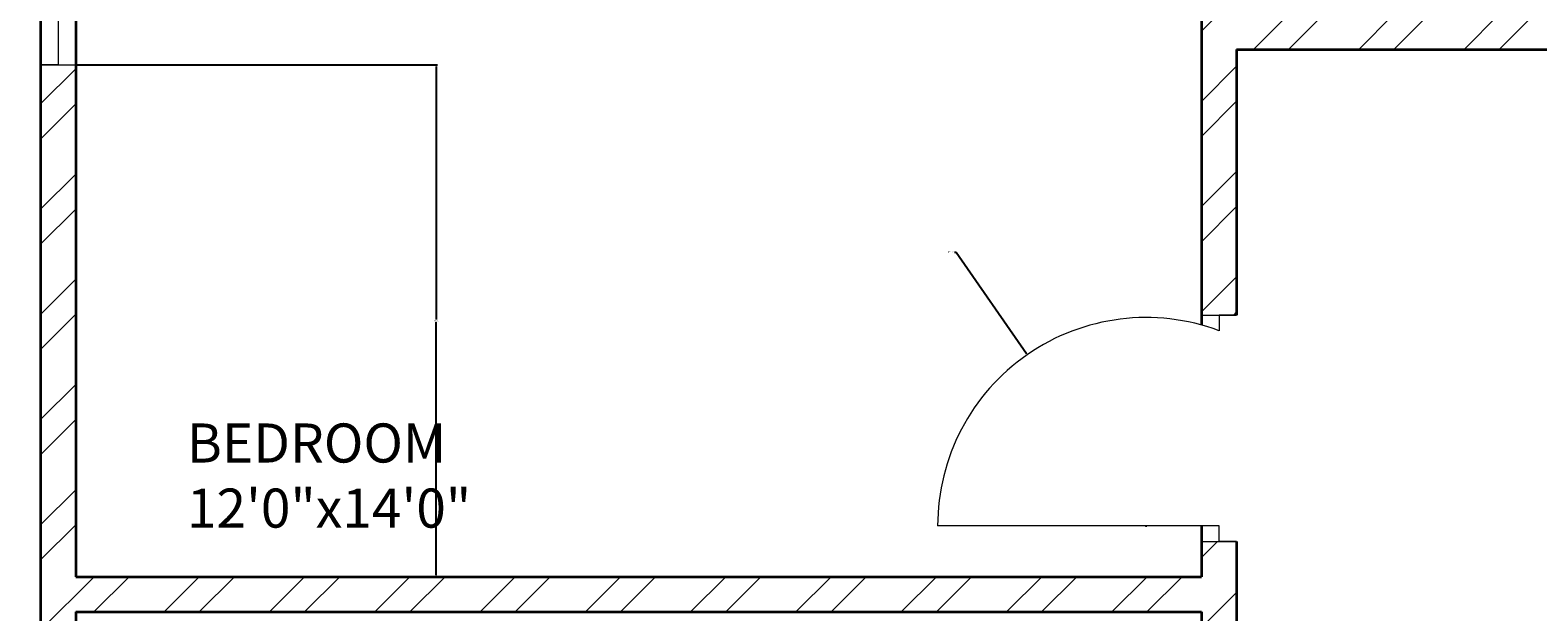
# Model space of a CAD drawing. Units: inches. Extents: x 392 to 1254, y 1207 to 2665.
# Tile 8 of 15: x 540 to 733, y 2052 to 2127. Entities that reach past the tile are written whole.
import ezdxf

# ---------------------------------------------------------------- set-up
doc = ezdxf.new("R2010")
doc.units = ezdxf.units.IN
for name, color, linetype, lineweight in [('A-ANNO-DIMS', 2, 'Continuous', 18), ('A-AREA-IDEN', 7, 'Continuous', 18), ('A-DOOR', 3, 'Continuous', 18), ('A-GLAZ', 4, 'Continuous', 18), ('A-WALL', 7, 'Continuous', 35), ('A-WALL-PATT', 252, 'Continuous', 13)]:
    doc.layers.add(name, color=color, linetype=linetype, lineweight=lineweight)
doc.styles.get("Standard").update_dxf_attribs({"font": 'arial.ttf'})
doc.dimstyles.get("Standard").update_dxf_attribs({"dimtxt": 0.18, "dimasz": 0.18, "dimexe": 0.18, "dimexo": 0.0625, "dimgap": 0.09, "dimtad": 0, "dimtih": 1, "dimtoh": 1, "dimdec": 4, "dimzin": 0, "dimdsep": 46, "dimtxsty": 'Standard', "dimcen": 0.09, "dimadec": 0, "dimazin": 0, "dimtfac": 1, "dimtdec": 4, "dimtofl": 0, "dimtmove": 0, "dimatfit": 3, "dimfxl": 1, "dimtolj": 1, "dimtzin": 0, "dimarcsym": 0})

# ---------------------------------------------------------------- blocks, each defined once
blk = doc.blocks.new('WIN-60-A')
for p, q in [((0, 60), (4.5, 60)), ((4.5, 60), (2.25, 60)), ((2.25, 60), (2.25, 0)), ((2.25, 0), (0, 0)), ((0, 0), (4.5, 0))]:
    blk.add_line(p, q)
blk = doc.blocks.new('*D26')
at = {"layer": 'A-ANNO-DIMS', "color": 0, "lineweight": -2, "transparency": 16777216}
for p, q in [((541.22, 2229.3), (495, 2229.3)), ((495.18, 2229.12), (495.18, 1819.98)), ((495.18, 1410.48), (495.18, 1819.61)), ((753.23, 1410.3), (495, 1410.3))]:
    blk.add_line(p, q, dxfattribs=at)
at = {"layer": 'A-ANNO-DIMS', "color": 0, "transparency": 16777216}
for points in [[(495.15, 2229.12), (495.21, 2229.12), (495.18, 2229.3)], [(495.15, 1410.48), (495.21, 1410.48), (495.18, 1410.3)]]:
    blk.add_solid(points, dxfattribs=at)
at = {"layer": 'Defpoints', "color": 0, "transparency": 16777216}
for p in [(495.18, 2229.3), (541.28, 2229.3), (753.29, 1410.3)]:
    blk.add_point(p, dxfattribs=at)
at = {"layer": 'A-ANNO-DIMS', "color": 0, "transparency": 16777216, "insert": (495.18, 1819.8), "char_height": 0.18, "attachment_point": 5}
blk.add_mtext('\\A1;819', dxfattribs=at)
blk = doc.blocks.new('*D35')
at = {"layer": 'A-ANNO-DIMS', "color": 0, "lineweight": -2, "transparency": 16777216}
for p, q in [((545.84, 2122.31), (592.06, 2122.31)), ((591.88, 2122.13), (591.88, 2089.73)), ((591.88, 2056.98), (591.88, 2089.37)), ((545.84, 2056.8), (592.06, 2056.8))]:
    blk.add_line(p, q, dxfattribs=at)
at = {"layer": 'A-ANNO-DIMS', "color": 0, "transparency": 16777216}
for points in [[(591.85, 2122.13), (591.91, 2122.13), (591.88, 2122.31)], [(591.85, 2056.98), (591.91, 2056.98), (591.88, 2056.8)]]:
    blk.add_solid(points, dxfattribs=at)
at = {"layer": 'Defpoints', "color": 0, "transparency": 16777216}
for p in [(545.78, 2122.31), (545.78, 2056.8), (591.88, 2056.8)]:
    blk.add_point(p, dxfattribs=at)
at = {"layer": 'A-ANNO-DIMS', "color": 0, "transparency": 16777216, "insert": (591.88, 2089.55), "char_height": 0.18, "attachment_point": 5}
blk.add_mtext('\\A1;65.51', dxfattribs=at)
blk = doc.blocks.new('*D94')
at = {"layer": 'A-ANNO-DIMS', "color": 0, "lineweight": -2, "transparency": 16777216}
for p, q in [((658.2, 2098.36), (658.38, 2098.36)), ((658.38, 2098.36), (667.39, 2085.37)), ((682.6, 2063.31), (682.78, 2063.31)), ((682.69, 2063.22), (682.69, 2063.4))]:
    blk.add_line(p, q, dxfattribs=at)
at = {"layer": 'A-ANNO-DIMS', "color": 0, "transparency": 16777216}
blk.add_solid([(667.42, 2085.38), (667.37, 2085.35), (667.5, 2085.22)], dxfattribs=at)
at = {"layer": 'Defpoints', "color": 0, "transparency": 16777216}
for p in [(667.5, 2085.22), (682.69, 2063.31)]:
    blk.add_point(p, dxfattribs=at)
at = {"layer": 'A-ANNO-DIMS', "color": 0, "transparency": 16777216, "insert": (657.72, 2098.36), "char_height": 0.18, "attachment_point": 5}
blk.add_mtext('\\A1;R26.66', dxfattribs=at)

msp = doc.modelspace()

# ---------------------------------------------------------------- hatches: boundary and pattern name
at = {"layer": 'A-WALL-PATT'}
h = msp.add_hatch(dxfattribs=at)
h.set_pattern_fill('ANSI32', color=256)
h.paths.add_polyline_path([(579.5309, 2227.0453), (579.5309, 2229.2953), (541.2807, 2229.2953), (541.2807, 2182.3091), (545.7807, 2182.3091), (545.7807, 2224.7953), (579.5309, 2224.7953)])
h.paths.add_polyline_path([(655.4442, 2229.2953), (627.5309, 2229.2953), (627.5309, 2224.7953), (655.4442, 2224.7953), (655.4442, 2227.0453)])
h.paths.add_polyline_path([(703.0758, 2229.2953), (678.5257, 2229.2953), (678.5257, 2227.0453), (678.5257, 2224.7953), (689.7807, 2224.7953), (689.7807, 2158.6973), (694.2807, 2158.6973), (694.2807, 2224.7953), (703.0758, 2224.7953)])
h.paths.add_polyline_path([(768.5767, 2229.2953), (727.0758, 2229.2953), (727.0758, 2224.7953), (742.2807, 2224.7953), (742.2807, 2128.7953), (694.2807, 2128.7953), (694.2807, 2134.0554), (689.7807, 2134.0554), (689.7807, 2090.2854), (694.2807, 2090.2854), (694.2807, 2124.2953), (742.2807, 2124.2953), (742.2807, 2052.2953), (795.2124, 2052.2953), (795.2124, 2054.5453), (795.2124, 2056.7953), (746.7807, 2056.7953), (746.7807, 2224.7953), (768.5767, 2224.7953)])
h.paths.add_polyline_path([(867.5089, 2229.2953), (804.5767, 2229.2953), (804.5767, 2224.7953), (830.7807, 2224.7953), (830.7807, 2056.7953), (826.9066, 2056.7953), (826.9066, 2052.2953), (830.7807, 2052.2953), (830.7807, 1886.6777, -0.01766664), (830.8602, 1884.2953), (835.0818, 1884.2953, -0.04411348), (835.2807, 1889.9369), (835.2807, 2052.2953), (839.418, 2052.2953), (839.418, 2056.7953), (835.2807, 2056.7953), (835.2807, 2224.7953), (867.5089, 2224.7953)])
h.paths.add_polyline_path([(939.8604, 2229.2953), (903.5089, 2229.2953), (903.5089, 2227.0453), (903.5089, 2224.7953), (919.2807, 2224.7953), (919.2807, 2056.7953), (870.6499, 2056.7953), (870.6499, 2052.2953), (923.7807, 2052.2953), (923.7807, 2124.2953), (971.7807, 2124.2953), (971.7807, 2089.7112), (974.0307, 2089.7112), (976.2807, 2089.7112), (976.2807, 2133.56), (974.0307, 2133.56), (971.7807, 2133.56), (971.7807, 2128.7953), (923.7807, 2128.7953), (923.7807, 2224.7953), (939.8604, 2224.7953)])
h.paths.add_polyline_path([(1124.7807, 2229.2953), (1009.403, 2229.2953), (1009.403, 2224.7953), (1120.2807, 2224.7953), (1120.2807, 2184.7605), (1124.7807, 2184.7605)])
h.paths.add_polyline_path([(1124.7807, 2124.7605), (1120.2807, 2124.7605), (1120.2807, 2056.7953), (976.2807, 2056.7953), (976.2807, 2061.471), (971.7807, 2061.471), (971.7807, 2047.7483), (974.0307, 2047.7483), (976.2807, 2047.7483), (976.2807, 2052.2953), (1120.2807, 2052.2953), (1120.2807, 1992.457), (1124.7807, 1992.457)])
h.paths.add_polyline_path([(1124.7807, 1932.457), (1122.5307, 1932.457), (1120.2807, 1932.457), (1120.2807, 1884.2953), (976.2807, 1884.2953), (976.2807, 2019.9536), (971.7807, 2019.9536), (971.7807, 1884.2953), (869.0911, 1884.2953), (869.0911, 1879.7953), (971.7807, 1879.7953), (1013.7807, 1879.7953), (1013.7807, 1831.7953), (971.7807, 1831.7953), (971.7807, 1822.3831), (974.0307, 1822.3831), (976.2807, 1822.3831), (976.2807, 1827.2953), (1013.7807, 1827.2953), (1025.6191, 1827.2953), (1025.6191, 1829.5453), (1025.6191, 1831.7953), (1018.2807, 1831.7953), (1018.2807, 1879.7953), (1120.2807, 1879.7953), (1120.2807, 1866.9192), (1124.7807, 1866.9192)])
h.paths.add_polyline_path([(1124.7807, 1842.9192), (1122.5307, 1842.9192), (1120.2807, 1842.9192), (1120.2807, 1831.7953), (1050.2021, 1831.7953), (1050.2021, 1827.2953), (1120.2807, 1827.2953), (1120.2807, 1781.4559), (1124.7807, 1781.4559)])
h.paths.add_polyline_path([(976.2807, 1790.8718), (971.7807, 1790.8718), (971.7807, 1648.3339), (976.2807, 1648.3339), (976.2807, 1654.7953), (1120.2807, 1654.7953), (1120.2807, 1626.3807), (1124.7807, 1626.3807), (1124.7807, 1721.4559), (1120.2807, 1721.4559), (1120.2807, 1659.2953), (976.2807, 1659.2953)])
h.paths.add_polyline_path([(1124.7807, 1566.3807), (1120.2807, 1566.3807), (1120.2807, 1486.7953), (1101.07, 1486.7953), (1101.07, 1482.2953), (1124.7807, 1482.2953)])
h.paths.add_polyline_path([(1041.07, 1484.5453), (1041.07, 1486.7953), (1006.2807, 1486.7953), (1006.2807, 1484.5453), (1006.2807, 1482.2953), (1041.07, 1482.2953)])
h.paths.add_polyline_path([(976.2807, 1617.5497), (974.0307, 1617.5497), (971.7807, 1617.5497), (971.7807, 1599.2953), (965.8041, 1599.2953), (965.8041, 1594.7953), (971.7807, 1594.7953), (971.7807, 1486.7953), (954.1249, 1486.7953), (954.1249, 1482.2953), (981.5717, 1482.2953), (981.5717, 1484.5453), (981.5717, 1486.7953), (976.2807, 1486.7953)])
h.paths.add_polyline_path([(930.1249, 1486.7953), (887.7807, 1486.7953), (887.7807, 1594.7953), (941.9141, 1594.7953), (941.9141, 1597.0453), (941.9141, 1599.2953), (887.7807, 1599.2953), (887.7807, 1659.2953), (863.5916, 1659.2953), (863.5916, 1654.7953), (883.2807, 1654.7953), (883.2807, 1438.7953), (782.7807, 1438.7953), (782.7807, 1486.7953), (782.7807, 1654.7953), (800.1309, 1654.7953), (800.1309, 1657.0453), (800.1309, 1659.2953), (778.2807, 1659.2953), (778.2807, 1599.2953), (721.7333, 1599.2953), (721.7333, 1597.0453), (721.7333, 1594.7953), (778.2807, 1594.7953), (778.2807, 1486.7953), (729.598, 1486.7953), (729.598, 1482.2953), (753.2885, 1482.2953), (753.2885, 1410.2953), (922.9852, 1410.2953), (922.9852, 1482.2953), (930.1249, 1482.2953)])
h.paths.add_polyline_path([(918.4852, 1482.2953), (918.4852, 1414.7953), (757.7885, 1414.7953), (757.7885, 1482.2953), (778.2807, 1482.2953), (778.2807, 1434.2953), (782.7807, 1434.2953), (887.7807, 1434.2953), (887.7807, 1438.7953), (887.7807, 1482.2953)], flags=16)
h.paths.add_polyline_path([(694.2807, 1594.7953), (700.4169, 1594.7953), (700.4169, 1597.0453), (700.4169, 1599.2953), (694.2807, 1599.2953), (694.2807, 1617.7503), (692.0307, 1617.7503), (689.7807, 1617.7503), (689.7807, 1486.7953), (682.7672, 1486.7953), (682.7672, 1482.2953), (705.598, 1482.2953), (705.598, 1484.5453), (705.598, 1486.7953), (694.2807, 1486.7953)])
h.paths.add_polyline_path([(545.7807, 1654.7953), (689.7807, 1654.7953), (689.7807, 1649.7691), (694.2807, 1649.7691), (694.2807, 1789.3981), (692.0307, 1789.3981), (689.7807, 1789.3981), (689.7807, 1659.2953), (545.7807, 1659.2953), (545.7807, 1714.4681), (543.5307, 1714.4681), (541.2807, 1714.4681), (541.2807, 1482.2953), (567.0628, 1482.2953), (567.0628, 1484.5453), (567.0628, 1486.7953), (545.7807, 1486.7953)])
h.paths.add_polyline_path([(545.7807, 1827.2953), (620.2247, 1827.2953), (620.2247, 1829.5453), (620.2247, 1831.7953), (545.7807, 1831.7953), (545.7807, 1846.8518), (541.2807, 1846.8518), (541.2807, 1774.4681), (545.7807, 1774.4681)])
h.paths.add_polyline_path([(797.0944, 1884.2953), (694.2807, 1884.2953), (694.2807, 2019.0288), (692.0307, 2019.0288), (689.7807, 2019.0288), (689.7807, 1884.2953), (545.7807, 1884.2953), (545.7807, 1951.8244), (541.2807, 1951.8244), (541.2807, 1870.8518), (543.5307, 1870.8518), (545.7807, 1870.8518), (545.7807, 1879.7953), (647.7807, 1879.7953), (647.7807, 1831.7953), (642.6413, 1831.7953), (642.6413, 1827.2953), (652.2807, 1827.2953), (689.7807, 1827.2953), (689.7807, 1821.0531), (694.2807, 1821.0531), (694.2807, 1831.7953), (652.2807, 1831.7953), (652.2807, 1879.7953), (797.0944, 1879.7953), (797.0944, 1882.0453)])
h.paths.add_polyline_path([(545.7807, 2122.3091), (541.2807, 2122.3091), (541.2807, 2011.8244), (543.5307, 2011.8244), (545.7807, 2011.8244), (545.7807, 2052.2953), (689.7807, 2052.2953), (689.7807, 2048.2048), (694.2807, 2048.2048), (694.2807, 2061.3129), (692.0307, 2061.3129), (689.7807, 2061.3129), (689.7807, 2056.7953), (545.7807, 2056.7953)])

# ---------------------------------------------------------------- linework, layer by layer
at = {"layer": 'A-DOOR'}
for p, q in [((689.7807, 2090.2854), (694.2807, 2090.2854)), ((694.2807, 2090.2854), (692.0307, 2090.2854)), ((692.0307, 2090.2854), (692.0307, 2088.2854)), ((692.0307, 2063.3129), (656.0307, 2063.3129)), ((692.0307, 2061.3129), (692.0307, 2063.3129)), ((689.7807, 2061.3129), (694.2807, 2061.3129)), ((694.2807, 2061.3129), (692.0307, 2061.3129))]:
    msp.add_line(p, q, dxfattribs=at)
msp.add_arc((682.6922, 2063.3129), 26.6615, 69.496743, 180, dxfattribs=at)
at = {"layer": 'A-WALL'}
for p, q in [((541.2807, 2229.2953), (541.2807, 1482.2953)), ((545.7807, 2224.7953), (545.7807, 2056.7953)), ((689.7807, 2134.0554), (689.7807, 2089.0148)), ((694.2807, 2124.2953), (742.2807, 2124.2953)), ((694.2807, 2124.2953), (694.2807, 2090.2854)), ((689.7807, 2063.3129), (689.7807, 2056.7953)), ((694.2807, 2061.3129), (694.2807, 2048.2048)), ((545.7807, 2056.7953), (689.7807, 2056.7953)), ((545.7807, 2052.2953), (689.7807, 2052.2953)), ((545.7807, 2052.2953), (545.7807, 1884.2953)), ((689.7807, 2052.2953), (689.7807, 2046.2048))]:
    msp.add_line(p, q, dxfattribs=at)

# ---------------------------------------------------------------- block references
at = {"layer": 'A-GLAZ'}
msp.add_blockref('WIN-60-A', (541.281, 2122.309), dxfattribs=at)

# ---------------------------------------------------------------- texts
at = {"layer": 'A-AREA-IDEN', "insert": (559.9889, 2076.4126), "char_height": 5, "attachment_point": 1}
msp.add_mtext_dynamic_manual_height_columns('BEDROOM\\P12\'0"x14\'0"', width=127.339145, gutter_width=12.5, heights=[0], dxfattribs=at)

# ---------------------------------------------------------------- dimensions: what is measured, and where the dimension line sits
at = {"layer": 'A-ANNO-DIMS'}
for base, p1, p2, angle, override, picture, middle in [((495.1807, 2229.2953), (753.2885, 1410.2953), (541.2807, 2229.2953), 90, {"dimdec": 0, "dimlfac": 1, "dimrnd": 0, "dimzin": 0, "dimdsep": 46, "dimlunit": 2}, '*D26', (495.1807, 1819.7953)), ((591.8807, 2056.7953), (545.7807, 2122.3091), (545.7807, 2056.7953), 270, {"dimdec": 2, "dimlfac": 1, "dimrnd": 0, "dimzin": 0, "dimdsep": 46, "dimlunit": 2}, '*D35', (591.8807, 2089.5522))]:
    dim = msp.add_linear_dim(base=base, p1=p1, p2=p2, angle=angle, dimstyle='Standard', override=override, dxfattribs=at)
    dim.commit()
    dim.dimension.update_dxf_attribs({"geometry": picture, "text_midpoint": middle})
dim = msp.add_radius_dim(center=(682.6922, 2063.3129), mpoint=(667.4961, 2085.2198), dimstyle='Standard', override={"dimdec": 2, "dimlfac": 1, "dimrnd": 0, "dimzin": 0, "dimdsep": 46, "dimlunit": 2}, dxfattribs=at)
dim.commit()
dim.dimension.update_dxf_attribs({"geometry": '*D94', "text_midpoint": (657.7187, 2098.364), "dimtype": 164})

doc.saveas('drawing.dxf')
